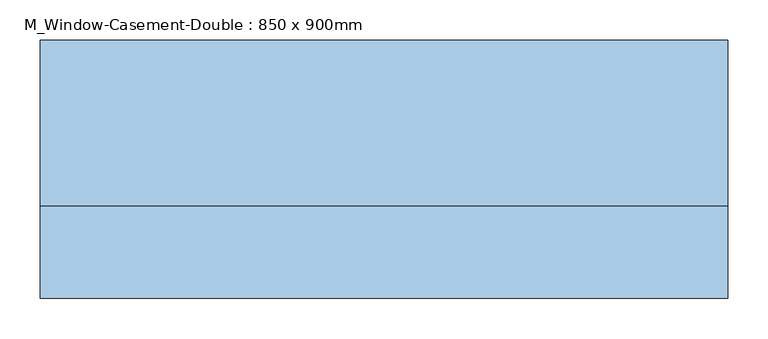
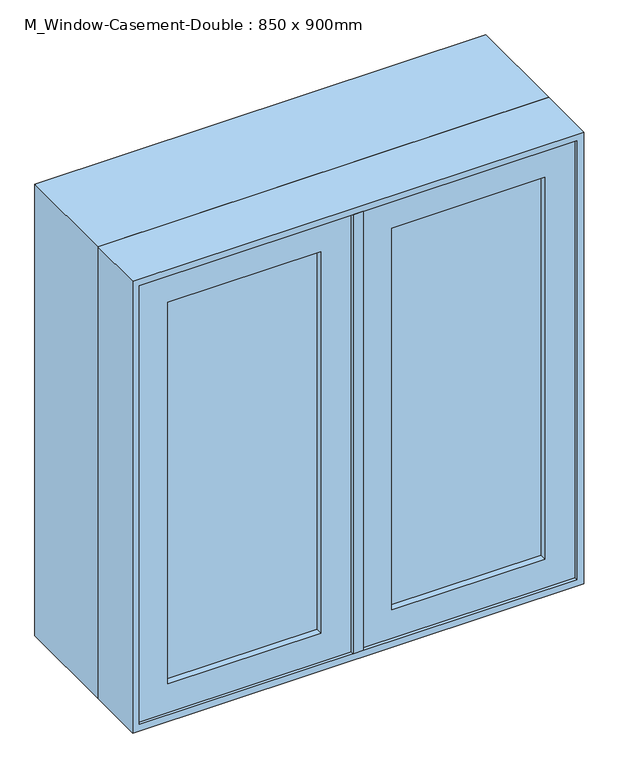
"""IFC4 building model written with IfcOpenShell, lengths in millimetres: window geometry, M_Window-Casement-Double : 850 x 900mm."""

from ifc_helpers import new_model, si_unit, frame, origin, place, context, project, spatial, polyline, outline, extrude, faceted_brep, source, transform, mapped, element, save


def m_window_casement_double_850_x_900mm_ced1a82e(model_context):
    return source(origin(), model_context, "Body", "SolidModel", [
        faceted_brep([(9.525, -169.05, 1787.3), (9.525, -118.25, 1787.3), (-9.525, -118.25, 1787.3), (-9.525, -169.05, 1787.3), (9.525, -169.05, 912.7), (-9.525, -169.05, 912.7), (-9.525, -118.25, 912.7), (9.525, -118.25, 912.7), (-9.525, -118.25, 1768.25), (-9.525, -118.25, 931.75), (-30.1625, -118.25, 1768.25), (-30.1625, -118.25, 931.75), (-30.1625, -54.75, 1768.25), (-30.1625, -54.75, 931.75), (30.1625, -54.75, 1768.25), (30.1625, -54.75, 931.75), (30.1625, -118.25, 1768.25), (30.1625, -118.25, 931.75), (9.525, -118.25, 1768.25), (9.525, -118.25, 931.75)], [[[0, 1, 2, 3]], [[4, 5, 6, 7]], [[3, 5, 4, 0]], [[2, 8, 9, 6, 5, 3]], [[8, 10, 11, 9]], [[10, 12, 13, 11]], [[12, 14, 15, 13]], [[14, 16, 17, 15]], [[16, 18, 19, 17]], [[0, 4, 7, 19, 18, 1]], [[8, 2, 1, 18]], [[19, 7, 6, 9]], [[9, 11, 13, 15, 17, 19]], [[18, 16, 14, 12, 10, 8]]]),
        extrude(outline(polyline([(-66.675, -150.0), (-355.15, -150.0), (-355.15, -143.65), (-66.675, -143.65), (-66.675, -150.0)])), frame((0.0, 0.0, 969.85), z_axis=(0.0, 0.0, 1.0), x_axis=(1.0, 0.0, 0.0)), (0.0, 0.0, 1.0), 760.3),
        extrude(outline(polyline([(-355.15, -130.95), (-66.675, -130.95), (-66.675, -137.3), (-355.15, -137.3), (-355.15, -130.95)])), frame((0.0, 0.0, 969.85), z_axis=(0.0, 0.0, 1.0), x_axis=(1.0, 0.0, 0.0)), (0.0, 0.0, 1.0), 760.3),
        extrude(outline(polyline([(355.15, -150.0), (66.675, -150.0), (66.675, -143.65), (355.15, -143.65), (355.15, -150.0)])), frame((0.0, 0.0, 969.85), z_axis=(0.0, 0.0, 1.0), x_axis=(1.0, 0.0, 0.0)), (0.0, 0.0, 1.0), 760.3),
        extrude(outline(polyline([(66.675, -130.95), (355.15, -130.95), (355.15, -137.3), (66.675, -137.3), (66.675, -130.95)])), frame((0.0, 0.0, 969.85), z_axis=(0.0, 0.0, 1.0), x_axis=(1.0, 0.0, 0.0)), (0.0, 0.0, 1.0), 760.3),
        extrude(outline(polyline([(1787.3, -9.525), (1787.3, -412.3), (912.7, -412.3), (912.7, -9.525), (1787.3, -9.525)]), holes=[polyline([(1730.15, -355.15), (1730.15, -66.675), (969.85, -66.675), (969.85, -355.15), (1730.15, -355.15)])]), frame((0.0, -162.7, 0.0), z_axis=(0.0, 1.0, 0.0), x_axis=(0.0, 0.0, 1.0)), (0.0, 0.0, 1.0), 44.45),
        extrude(outline(polyline([(912.7, 9.525), (912.7, 412.3), (1787.3, 412.3), (1787.3, 9.525), (912.7, 9.525)]), holes=[polyline([(969.85, 355.15), (969.85, 66.675), (1730.15, 66.675), (1730.15, 355.15), (969.85, 355.15)])]), frame((0.0, -162.7, 0.0), z_axis=(0.0, 1.0, 0.0), x_axis=(0.0, 0.0, 1.0)), (0.0, 0.0, 1.0), 44.45),
        extrude(outline(polyline([(1800.0, -425.0), (900.0, -425.0), (900.0, 425.0), (1800.0, 425.0), (1800.0, -425.0)]), holes=[polyline([(1780.95, 405.95), (919.05, 405.95), (919.05, -405.95), (1780.95, -405.95), (1780.95, 405.95)])]), frame((0.0, -54.75, 0.0), z_axis=(0.0, 1.0, 0.0), x_axis=(0.0, 0.0, 1.0)), (0.0, 0.0, 1.0), 204.75),
        faceted_brep([(393.25, -118.25, 1768.25), (-393.25, -118.25, 1768.25), (-393.25, -54.75, 1768.25), (393.25, -54.75, 1768.25), (412.3, -169.05, 1787.3), (-412.3, -169.05, 1787.3), (-412.3, -118.25, 1787.3), (412.3, -118.25, 1787.3), (425.0, -54.75, 1800.0), (-425.0, -54.75, 1800.0), (-425.0, -169.05, 1800.0), (425.0, -169.05, 1800.0), (-393.25, -118.25, 931.75), (-393.25, -54.75, 931.75), (-412.3, -169.05, 912.7), (-412.3, -118.25, 912.7), (-425.0, -54.75, 900.0), (-425.0, -169.05, 900.0), (393.25, -118.25, 931.75), (393.25, -54.75, 931.75), (412.3, -169.05, 912.7), (412.3, -118.25, 912.7), (425.0, -54.75, 900.0), (425.0, -169.05, 900.0)], [[[0, 1, 2, 3]], [[4, 5, 6, 7]], [[8, 9, 10, 11]], [[1, 12, 13, 2]], [[5, 14, 15, 6]], [[9, 16, 17, 10]], [[12, 18, 19, 13]], [[14, 20, 21, 15]], [[16, 22, 23, 17]], [[9, 8, 22, 16], [3, 2, 13, 19]], [[18, 0, 3, 19]], [[7, 6, 15, 21], [1, 0, 18, 12]], [[20, 4, 7, 21]], [[22, 8, 11, 23]], [[11, 10, 17, 23], [5, 4, 20, 14]]]),
    ])


if __name__ == "__main__":
    model = new_model("IFC4")
    model_context = context("Model", 3, world=origin())
    ifc_project = project(units=[si_unit("LENGTHUNIT", "METRE", prefix="MILLI")], contexts=[model_context])
    site = spatial("IfcSite", under=ifc_project)
    building = spatial("IfcBuilding", under=site)
    placement = place(None, origin())
    m_window_casement_double_850_x_900mm_shape = m_window_casement_double_850_x_900mm_ced1a82e(model_context)
    element("IfcWindow", 1, ObjectType="M_Window-Casement-Double : 850 x 900mm", at=placement, inside=building, context=model_context, shape_type="MappedRepresentation", body=[
        mapped(m_window_casement_double_850_x_900mm_shape, transform((0.0, 0.0, 0.0), x_axis=(1.0, 0.0, 0.0), y_axis=(0.0, 1.0, 0.0), z_axis=(0.0, 0.0, 1.0))),
    ])
    save(model, "model.ifc")

# Revit data of these elements
# Type "M_Window-Casement-Double : 850 x 900mm"
#   Type Mark = "23"
#   Fire Rating = "0.5h"
#   Assembly Code = "B2020100"
#   Analytic Construction = "Double glazing - domestic"
#   Frame Extension [instance default] = 6.35 mm
#   Window Inset [instance default] = 0 mm
#   Wall Thickness [instance default] = 150 mm
#   Interior Wall Closure [instance default] = 54.75 mm
#   Half Width = 425 mm
#   Visual Light Transmittance = 0.81
#   Thermal Resistance (R) = 0.319569 (m²·K)/W
#   Solar Heat Gain Coefficient = 0.76
#   Rough Width = 865 mm
#   Rough Height = 915 mm
#   Height = 900 mm
#   Heat Transfer Coefficient (U) = 3.12929 W/(m²·K)
#   Exterior Wall Closure [instance default] = 31.8 mm
#   Extension Jamb [instance default] = 54.75 mm
#   Default Sill Height = 900 mm
#   Width = 850 mm
#   Define Thermal Properties by = 0
#   Muntin Visibility = yes
#   Interior Trim Visibility [instance default] = yes
#   Exterior Trim Visibility [instance default] = yes
#   Extension Jamb Visibility [instance default] = yes
#   Interior Trim Material = Wood - Stained
#   Muntin Pattern = M_Muntin Pattern_2x2 : M_Muntin Pattern_2x2
#   Interior Trim = M_Trim-Window-Interior-Flat : Picture Frame
#   Interior Frame Material = Wood - Stained
#   Glass Panel Material = Glass
#   Exterior Trim Material = Clad - White
#   Exterior Trim = M_Trim-Window-Exterior-Flat : with Sill
#   Exterior Frame Material = Clad - White
#   Wall Closure = (empty or 0)
# Element 1 (IfcWindow, "M_Window-Casement-Double : 850 x 900mm")
#   Wall Thickness = 300 mm
#   Extension Jamb = 204.75 mm
#   Materials on its faces: "Wood - Stained", "Glass", "Clad - White"
# Materials
#   "Wood - Stained": class "Wood", colour RGB 224 178 126, transparency 0, Cost = 0
#   "Glass": class "Glass", colour RGB 0 128 192, transparency 0.9, Description = "Soda Lime Glass", Cost = 0
#   "Clad - White": class "Wood", colour RGB 242 242 238, transparency 0, Cost = 0
